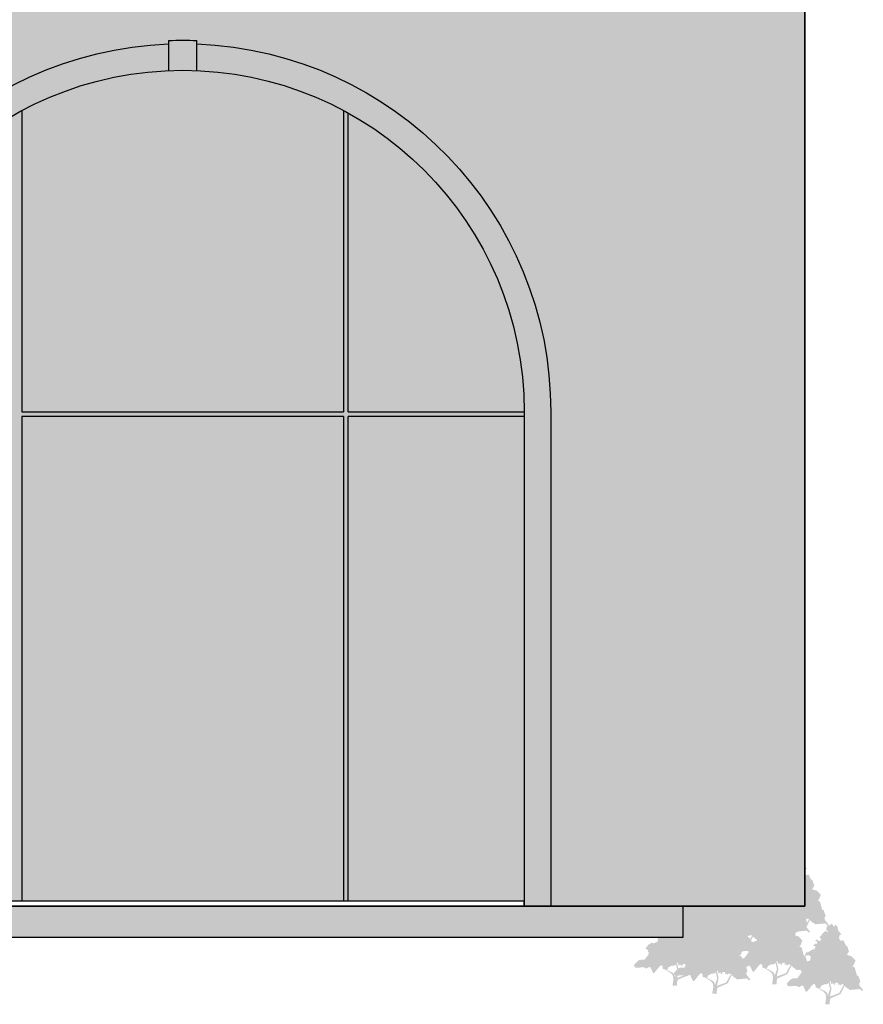
# Model space of a CAD drawing. Units: feet. Extents: x 2368 to 3224, y 836 to 1229.
# Tile 7 of 9: x 2603 to 2728, y 839 to 985. Entities that reach past the tile are written whole.
import ezdxf

# ---------------------------------------------------------------- set-up
doc = ezdxf.new("R2010")
doc.units = ezdxf.units.FT
for name, color, linetype, lineweight in [('A-ELEV', 7, 'Continuous', 25), ('A-ELEV-PATT', 8, 'Continuous', 13), ('L-PLNT', 3, 'Continuous', 13)]:
    doc.layers.add(name, color=color, linetype=linetype, lineweight=lineweight)

msp = doc.modelspace()

# ---------------------------------------------------------------- hatches: boundary and pattern name
at = {"layer": 'A-ELEV-PATT'}
h = msp.add_hatch(color=256, dxfattribs=at)
h.dxf.hatch_style = 1
h.paths.add_polyline_path([(2582.11, 1191.22), (2544.98, 1191.22), (2544.98, 1108.75), (2582.11, 1108.75)])
h.paths.add_polyline_path([(2653.72, 1191.22), (2584.6, 1191.22), (2584.6, 1108.75), (2653.72, 1108.75)])
h.paths.add_polyline_path([(2693.73, 1191.22), (2656.21, 1191.22), (2656.21, 1108.75), (2693.73, 1108.75)])
h.paths.add_polyline_path([(2653.72, 1099.51), (2584.6, 1099.51), (2584.6, 1040.78), (2653.72, 1040.78)])
h.paths.add_polyline_path([(2693.73, 1099.51), (2656.21, 1099.51), (2656.21, 1040.78), (2693.73, 1040.78)])
h.paths.add_polyline_path([(2582.11, 1099.51), (2544.98, 1099.51), (2544.98, 1040.78), (2582.11, 1040.78)])
h.paths.add_polyline_path([(2582.11, 1036.77), (2544.98, 1036.77), (2544.98, 1033.48), (2582.11, 1033.48)])
h.paths.add_polyline_path([(2582.11, 1033.11), (2544.98, 1033.11), (2544.98, 1029.83), (2582.11, 1029.83)])
h.paths.add_polyline_path([(2582.11, 1029.46), (2544.98, 1029.46), (2544.98, 1026.18), (2582.11, 1026.18)])
h.paths.add_polyline_path([(2582.11, 1025.81), (2544.98, 1025.81), (2544.98, 1022.52), (2582.11, 1022.52)])
h.paths.add_polyline_path([(2582.11, 1022.15), (2544.98, 1022.15), (2544.98, 1018.87), (2582.11, 1018.87)])
h.paths.add_polyline_path([(2582.11, 1018.5), (2544.98, 1018.5), (2544.98, 1015.21), (2582.11, 1015.21)])
h.paths.add_polyline_path([(2582.11, 1007.53), (2544.98, 1007.53), (2544.98, 1006.11), (2582.11, 1006.11)])
h.paths.add_polyline_path([(2582.11, 1011.19), (2544.98, 1011.19), (2544.98, 1007.9), (2582.11, 1007.9)])
h.paths.add_polyline_path([(2582.11, 1014.84), (2544.98, 1014.84), (2544.98, 1011.56), (2582.11, 1011.56)])
h.paths.add_polyline_path([(2619.49, 1007.53), (2584.6, 1007.53), (2584.6, 1006.11), (2619.49, 1006.11)])
h.paths.add_polyline_path([(2619.49, 1011.19), (2584.6, 1011.19), (2584.6, 1007.9), (2619.49, 1007.9)])
h.paths.add_polyline_path([(2619.49, 1014.84), (2584.6, 1014.84), (2584.6, 1011.56), (2619.49, 1011.56)])
h.paths.add_polyline_path([(2619.49, 1018.5), (2584.6, 1018.5), (2584.6, 1015.21), (2619.49, 1015.21)])
h.paths.add_polyline_path([(2619.49, 1022.15), (2584.6, 1022.15), (2584.6, 1018.87), (2619.49, 1018.87)])
h.paths.add_polyline_path([(2619.49, 1025.81), (2584.6, 1025.81), (2584.6, 1022.52), (2619.49, 1022.52)])
h.paths.add_polyline_path([(2619.49, 1029.46), (2584.6, 1029.46), (2584.6, 1026.18), (2619.49, 1026.18)])
h.paths.add_polyline_path([(2619.49, 1033.11), (2584.6, 1033.11), (2584.6, 1029.83), (2619.49, 1029.83)])
h.paths.add_polyline_path([(2619.49, 1036.77), (2584.6, 1036.77), (2584.6, 1033.48), (2619.49, 1033.48)])
h.paths.add_polyline_path([(2582.11, 1040.06), (2544.98, 1040.06), (2544.98, 1037.14), (2582.11, 1037.14)])
h.paths.add_polyline_path([(2619.49, 1040.06), (2584.6, 1040.06), (2584.6, 1037.14), (2619.49, 1037.14)])
h.paths.add_polyline_path([(2653.72, 1040.06), (2620.43, 1040.06), (2620.43, 1037.14), (2653.72, 1037.14)])
h.paths.add_polyline_path([(2653.72, 1036.77), (2620.43, 1036.77), (2620.43, 1033.48), (2653.72, 1033.48)])
h.paths.add_polyline_path([(2653.72, 1033.11), (2620.43, 1033.11), (2620.43, 1029.83), (2653.72, 1029.83)])
h.paths.add_polyline_path([(2653.72, 1029.46), (2620.43, 1029.46), (2620.43, 1026.18), (2653.72, 1026.18)])
h.paths.add_polyline_path([(2653.72, 1025.81), (2620.43, 1025.81), (2620.43, 1022.52), (2653.72, 1022.52)])
h.paths.add_polyline_path([(2653.72, 1022.15), (2620.43, 1022.15), (2620.43, 1018.87), (2653.72, 1018.87)])
h.paths.add_polyline_path([(2653.72, 1018.5), (2620.43, 1018.5), (2620.43, 1015.21), (2653.72, 1015.21)])
h.paths.add_polyline_path([(2653.72, 1011.19), (2620.43, 1011.19), (2620.43, 1007.9), (2653.72, 1007.9)])
h.paths.add_polyline_path([(2653.72, 1014.84), (2620.43, 1014.84), (2620.43, 1011.56), (2653.72, 1011.56)])
h.paths.add_polyline_path([(2653.72, 1007.53), (2620.43, 1007.53), (2620.43, 1006.11), (2653.72, 1006.11)])
h.paths.add_polyline_path([(2693.73, 1007.53), (2656.21, 1007.53), (2656.21, 1006.11), (2693.73, 1006.11)])
h.paths.add_polyline_path([(2693.73, 1011.19), (2656.21, 1011.19), (2656.21, 1007.9), (2693.73, 1007.9)])
h.paths.add_polyline_path([(2693.73, 1014.84), (2656.21, 1014.84), (2656.21, 1011.56), (2693.73, 1011.56)])
h.paths.add_polyline_path([(2693.73, 1018.5), (2656.21, 1018.5), (2656.21, 1015.21), (2693.73, 1015.21)])
h.paths.add_polyline_path([(2693.73, 1022.15), (2656.21, 1022.15), (2656.21, 1018.87), (2693.73, 1018.87)])
h.paths.add_polyline_path([(2693.73, 1025.81), (2656.21, 1025.81), (2656.21, 1022.52), (2693.73, 1022.52)])
h.paths.add_polyline_path([(2693.73, 1029.46), (2656.21, 1029.46), (2656.21, 1026.18), (2693.73, 1026.18)])
h.paths.add_polyline_path([(2693.73, 1033.11), (2656.21, 1033.11), (2656.21, 1029.83), (2693.73, 1029.83)])
h.paths.add_polyline_path([(2693.73, 1040.06), (2656.21, 1040.06), (2656.21, 1037.14), (2693.73, 1037.14)])
h.paths.add_polyline_path([(2693.73, 1036.77), (2656.21, 1036.77), (2656.21, 1033.48), (2693.73, 1033.48)])
h.paths.add_polyline_path([(2510.02, 968.65), (2451.35, 968.65), (2451.35, 916.99), (2510.02, 916.99)])
h.paths.add_polyline_path([(2510.02, 916.99), (2470.8, 916.99), (2470.8, 861.76), (2510.02, 861.76)])
h.paths.add_polyline_path([(2650.82, 971.36, 0.250141), (2603.19, 971.36), (2603.19, 926.73), (2650.82, 926.73)])
h.paths.add_polyline_path([(2651.5, 971), (2651.5, 926.73), (2677.6, 926.73, 0.272847)])
h.paths.add_polyline_path([(2677.6, 926.06), (2651.5, 926.06), (2651.5, 854.24), (2677.6, 854.24)])
h.paths.add_polyline_path([(2650.82, 926.06), (2603.19, 926.06), (2603.19, 854.24), (2650.82, 854.24)])
h.paths.add_polyline_path([(2602.51, 971, 0.272847), (2576.42, 926.73), (2602.51, 926.73)])
h.paths.add_polyline_path([(2602.51, 926.06), (2576.42, 926.06), (2576.42, 854.24), (2602.51, 854.24)])
h = msp.add_hatch(color=256, dxfattribs=at)
h.dxf.hatch_style = 1
h.paths.add_polyline_path([(2624.92, 981.22), (2624.92, 981.73, -0.018787), (2629.09, 981.73), (2629.09, 981.22, -0.403049), (2681.53, 926.73), (2681.53, 853.51), (2701.14, 853.51), (2719.16, 853.51), (2719.16, 987.86), (2694.93, 987.86), (2544.98, 987.86), (2510.02, 987.86), (2510.02, 853.51), (2520.58, 853.51), (2520.05, 853.96), (2521, 855.17), (2521.51, 855.27), (2521.73, 855.83), (2522.31, 855.46), (2523.63, 855.92), (2523.84, 857.04), (2523.12, 857.51), (2521.95, 857.23), (2522.6, 858.63), (2522.68, 858.26), (2523.55, 858.73), (2524.28, 859.19), (2524.94, 859.29), (2525.23, 860.22), (2524.5, 860.32), (2525.17, 860.97), (2525.74, 860.88), (2525.67, 861.62), (2525.16, 861.72), (2525.3, 862.09), (2525.67, 862.19), (2526.32, 861.72), (2526.98, 862.19), (2526.47, 863.03), (2526.98, 863.31), (2526.98, 863.59), (2528.51, 865.09), (2528.51, 865.74), (2528.95, 866.58), (2529.53, 866.48), (2530.04, 866.95), (2530.41, 866.77), (2530.48, 866.3), (2530.77, 866.11), (2531.28, 866.67), (2531.86, 866.03), (2532.01, 864.99), (2533.1, 863.68), (2532.52, 863.68), (2532.3, 862.65), (2532.67, 861.9), (2533.18, 861.9), (2533.61, 862), (2534.34, 860.41), (2534.71, 860.41), (2535.29, 858.63), (2534.63, 857.61), (2536.09, 857.14), (2537.26, 855.92), (2536.52, 854.02), (2536.97, 853.96), (2537.09, 853.51), (2572.48, 853.51), (2572.48, 926.73, -0.403049)])
h.paths.add_polyline_path([(2536.7, 926.19), (2536.7, 904.71), (2529.87, 904.71), (2529.87, 926.19)], flags=16)
h = msp.add_hatch(color=256, dxfattribs=at)
h.dxf.hatch_style = 1
h.paths.add_polyline_path([(2624.92, 981.22, 0.403049), (2572.48, 926.73), (2572.48, 853.51), (2576.42, 853.51), (2576.42, 926.73, -0.402184), (2624.92, 977.28)])
h.paths.add_polyline_path([(2629.09, 981.22), (2629.09, 977.28, -0.402184), (2677.6, 926.73), (2677.6, 853.51), (2681.53, 853.51), (2681.53, 926.73, 0.403049)])
h.paths.add_polyline_path([(2629.09, 981.22), (2629.09, 981.73, 0.018787), (2624.92, 981.73), (2624.92, 977.28, -0.020626), (2629.09, 977.28)])
h = msp.add_hatch(color=256, dxfattribs=at)
h.dxf.hatch_style = 1
h.paths.add_polyline_path([(2603.19, 971.36, 0.00378), (2602.51, 971), (2602.51, 926.73), (2576.42, 926.73), (2576.42, 926.06), (2602.51, 926.06), (2602.51, 854.24), (2603.19, 854.24), (2603.19, 926.06), (2650.82, 926.06), (2650.82, 854.24), (2651.5, 854.24), (2651.5, 926.06), (2677.6, 926.06), (2677.6, 926.73), (2651.5, 926.73), (2651.5, 971, 0.00378), (2650.82, 971.36), (2650.82, 926.73), (2603.19, 926.73)])
h = msp.add_hatch(color=256, dxfattribs=at)
h.dxf.hatch_style = 1
h.paths.add_polyline_path([(2701.14, 853.51), (2538.51, 853.51), (2538.51, 848.93), (2701.14, 848.93)])
at = {"layer": 'L-PLNT'}
h = msp.add_hatch(color=256, dxfattribs=at)
h.dxf.hatch_style = 1
h.paths.add_polyline_path([(2709.04, 864.51), (2707.88, 865.72), (2706.42, 866.19), (2707.07, 867.22), (2706.49, 869), (2706.13, 869), (2705.4, 870.58), (2704.96, 870.49), (2704.45, 870.49), (2704.09, 871.24), (2704.3, 872.27), (2704.89, 872.27), (2703.79, 873.58), (2703.65, 874.61), (2703.06, 875.26), (2702.55, 874.7), (2702.26, 874.88), (2702.19, 875.35), (2701.83, 875.54), (2701.31, 875.07), (2700.73, 875.16), (2700.29, 874.32), (2700.29, 873.58), (2700.88, 873.3), (2700.44, 873.01), (2700, 873.39), (2698.76, 872.17), (2698.76, 871.89), (2698.25, 871.61), (2698.4, 871.33), (2698.76, 870.77), (2698.11, 870.3), (2697.45, 870.77), (2697.09, 870.68), (2696.94, 870.3), (2697.45, 870.21), (2697.52, 869.46), (2696.95, 869.56), (2696.28, 868.9), (2697.01, 868.81), (2696.72, 867.87), (2696.07, 867.78), (2695.34, 867.31), (2694.46, 866.85), (2694.39, 867.22), (2693.73, 865.82), (2694.9, 866.1), (2695.63, 865.63), (2695.41, 864.51), (2694.1, 864.04), (2693.51, 864.42), (2693.29, 863.85), (2692.78, 863.76), (2692.35, 863.2), (2691.84, 862.55), (2692.49, 861.99), (2692.93, 862.27), (2692.44, 861.45), (2692.79, 861.49), (2692.74, 860.76), (2691.54, 859.18), (2690.09, 859.09), (2689.43, 858.71), (2688.34, 857.5), (2688.77, 856.75), (2691.47, 856.84), (2691.98, 856.47), (2693.22, 857.03), (2694.1, 855.16), (2694.46, 855.16), (2696.14, 857.22), (2696.65, 857.5), (2697.01, 857.03), (2697.01, 856.38), (2697.6, 856.19), (2698.4, 856.19), (2698.69, 856.84), (2699.64, 857.31), (2700.59, 857.41), (2701.02, 857.78), (2701.1, 857.87), (2701.31, 858.34), (2701.61, 858.15), (2701.83, 857.41), (2702.34, 857.69), (2702.48, 857.5), (2702.63, 857.03), (2703.14, 857.87), (2703.65, 857.87), (2703.87, 857.5), (2703.65, 857.12), (2704.23, 857.31), (2704.45, 857.03), (2704.96, 857.41), (2705.47, 857.22), (2706.49, 856.19), (2706.93, 856), (2707.29, 855.63), (2710.36, 855.91), (2710.94, 855.35), (2711.38, 855.54), (2710.21, 857.03), (2710.14, 857.59), (2710.5, 858.15), (2709.85, 859.93), (2709.48, 859.93), (2708.75, 862.55), (2708.02, 862.64), (2708.46, 863.01)])
h = msp.add_hatch(color=256, dxfattribs=at)
h.dxf.hatch_style = 1
h.paths.add_polyline_path([(2711.33, 856.68), (2710.76, 857.28), (2710.04, 857.51), (2710.36, 858.02), (2710.08, 858.9), (2709.9, 858.9), (2709.54, 859.68), (2709.32, 859.63), (2709.07, 859.63), (2708.89, 860), (2709, 860.51), (2709.29, 860.51), (2708.75, 861.15), (2708.67, 861.67), (2708.39, 861.98), (2708.13, 861.71), (2707.99, 861.8), (2707.96, 862.03), (2707.78, 862.12), (2707.52, 861.89), (2707.24, 861.94), (2707.02, 861.52), (2707.02, 861.15), (2707.31, 861.02), (2707.09, 860.88), (2706.88, 861.06), (2706.27, 860.46), (2706.27, 860.33), (2706.01, 860.19), (2706.09, 860.05), (2706.27, 859.77), (2705.94, 859.54), (2705.62, 859.77), (2705.44, 859.73), (2705.37, 859.54), (2705.62, 859.5), (2705.65, 859.13), (2705.37, 859.17), (2705.04, 858.85), (2705.4, 858.8), (2705.26, 858.34), (2704.94, 858.3), (2704.58, 858.07), (2704.14, 857.84), (2704.11, 858.02), (2703.79, 857.33), (2704.36, 857.47), (2704.72, 857.24), (2704.61, 856.68), (2703.97, 856.45), (2703.68, 856.64), (2703.57, 856.36), (2703.32, 856.32), (2703.1, 856.04), (2702.85, 855.72), (2703.17, 855.44), (2703.39, 855.58), (2703.15, 855.18), (2703.32, 855.2), (2703.3, 854.84), (2702.71, 854.06), (2701.99, 854.01), (2701.66, 853.83), (2701.13, 853.23), (2701.34, 852.86), (2702.67, 852.91), (2702.92, 852.72), (2703.53, 853), (2703.97, 852.08), (2704.14, 852.08), (2704.97, 853.09), (2705.22, 853.23), (2705.4, 853), (2705.4, 852.68), (2705.69, 852.58), (2706.09, 852.58), (2706.23, 852.91), (2706.7, 853.14), (2707.16, 853.18), (2707.38, 853.37), (2707.42, 853.41), (2707.52, 853.64), (2707.67, 853.55), (2707.78, 853.18), (2708.03, 853.32), (2708.1, 853.23), (2708.17, 853), (2708.42, 853.41), (2708.67, 853.41), (2708.78, 853.23), (2708.67, 853.04), (2708.96, 853.14), (2709.07, 853), (2709.32, 853.18), (2709.57, 853.09), (2710.08, 852.58), (2710.29, 852.49), (2710.47, 852.31), (2711.98, 852.45), (2712.27, 852.17), (2712.48, 852.26), (2711.91, 853), (2711.87, 853.27), (2712.05, 853.55), (2711.73, 854.43), (2711.55, 854.43), (2711.19, 855.72), (2710.83, 855.76), (2711.05, 855.95)])
h = msp.add_hatch(color=256, dxfattribs=at)
h.dxf.hatch_style = 1
h.paths.add_polyline_path([(2720.19, 856.88), (2719.61, 857.48), (2718.89, 857.71), (2719.22, 858.22), (2718.93, 859.09), (2718.75, 859.09), (2718.39, 859.88), (2718.18, 859.83), (2717.92, 859.83), (2717.74, 860.2), (2717.85, 860.71), (2718.14, 860.71), (2717.6, 861.35), (2717.53, 861.86), (2717.24, 862.18), (2716.99, 861.9), (2716.85, 862), (2716.81, 862.23), (2716.63, 862.32), (2716.38, 862.09), (2716.09, 862.13), (2715.88, 861.72), (2715.88, 861.35), (2716.16, 861.21), (2715.95, 861.07), (2715.73, 861.26), (2715.12, 860.66), (2715.12, 860.52), (2714.87, 860.38), (2714.94, 860.25), (2715.12, 859.97), (2714.8, 859.74), (2714.47, 859.97), (2714.29, 859.92), (2714.22, 859.74), (2714.47, 859.69), (2714.51, 859.32), (2714.23, 859.37), (2713.9, 859.05), (2714.26, 859), (2714.11, 858.54), (2713.79, 858.49), (2713.43, 858.26), (2713, 858.03), (2712.96, 858.22), (2712.64, 857.53), (2713.22, 857.66), (2713.57, 857.43), (2713.47, 856.88), (2712.82, 856.65), (2712.53, 856.84), (2712.42, 856.56), (2712.17, 856.51), (2711.96, 856.24), (2711.71, 855.91), (2712.03, 855.64), (2712.24, 855.78), (2712, 855.37), (2712.18, 855.4), (2712.15, 855.03), (2711.56, 854.25), (2710.84, 854.21), (2710.52, 854.02), (2709.98, 853.43), (2710.2, 853.06), (2711.53, 853.1), (2711.78, 852.92), (2712.39, 853.19), (2712.82, 852.27), (2713, 852.27), (2713.83, 853.29), (2714.08, 853.43), (2714.26, 853.19), (2714.26, 852.87), (2714.55, 852.78), (2714.94, 852.78), (2715.08, 853.1), (2715.55, 853.33), (2716.02, 853.38), (2716.23, 853.56), (2716.27, 853.61), (2716.38, 853.84), (2716.52, 853.75), (2716.63, 853.38), (2716.88, 853.52), (2716.95, 853.43), (2717.03, 853.19), (2717.28, 853.61), (2717.53, 853.61), (2717.64, 853.43), (2717.53, 853.24), (2717.82, 853.33), (2717.92, 853.19), (2718.18, 853.38), (2718.43, 853.29), (2718.93, 852.78), (2719.15, 852.69), (2719.33, 852.5), (2720.84, 852.64), (2721.12, 852.37), (2721.34, 852.46), (2720.76, 853.19), (2720.73, 853.47), (2720.91, 853.75), (2720.58, 854.62), (2720.4, 854.62), (2720.04, 855.91), (2719.69, 855.96), (2719.9, 856.14)])
h = msp.add_hatch(color=256, dxfattribs=at)
h.dxf.hatch_style = 1
h.paths.add_polyline_path([(2721.54, 855.2), (2720.97, 855.8), (2720.25, 856.03), (2720.57, 856.54), (2720.28, 857.42), (2720.1, 857.42), (2719.75, 858.2), (2719.53, 858.15), (2719.28, 858.15), (2719.1, 858.52), (2719.21, 859.03), (2719.49, 859.03), (2718.95, 859.67), (2718.88, 860.19), (2718.6, 860.5), (2718.34, 860.23), (2718.2, 860.32), (2718.16, 860.55), (2717.98, 860.64), (2717.73, 860.41), (2717.44, 860.46), (2717.23, 860.04), (2717.23, 859.67), (2717.52, 859.54), (2717.3, 859.4), (2717.09, 859.58), (2716.47, 858.98), (2716.47, 858.84), (2716.22, 858.71), (2716.29, 858.57), (2716.47, 858.29), (2716.15, 858.06), (2715.83, 858.29), (2715.65, 858.25), (2715.58, 858.06), (2715.83, 858.01), (2715.86, 857.65), (2715.58, 857.69), (2715.25, 857.37), (2715.61, 857.32), (2715.47, 856.86), (2715.14, 856.82), (2714.79, 856.59), (2714.35, 856.36), (2714.32, 856.54), (2713.99, 855.85), (2714.57, 855.99), (2714.93, 855.76), (2714.82, 855.2), (2714.17, 854.97), (2713.89, 855.16), (2713.78, 854.88), (2713.53, 854.84), (2713.31, 854.56), (2713.06, 854.24), (2713.38, 853.96), (2713.6, 854.1), (2713.35, 853.7), (2713.53, 853.72), (2713.51, 853.36), (2712.92, 852.58), (2712.2, 852.53), (2711.87, 852.35), (2711.33, 851.75), (2711.55, 851.38), (2712.88, 851.43), (2713.13, 851.24), (2713.74, 851.52), (2714.17, 850.6), (2714.35, 850.6), (2715.18, 851.61), (2715.43, 851.75), (2715.61, 851.52), (2715.61, 851.19), (2715.9, 851.1), (2716.29, 851.1), (2716.44, 851.43), (2716.91, 851.66), (2717.37, 851.7), (2717.59, 851.89), (2717.62, 851.93), (2717.73, 852.16), (2717.88, 852.07), (2717.98, 851.7), (2718.24, 851.84), (2718.31, 851.75), (2718.38, 851.52), (2718.63, 851.93), (2718.88, 851.93), (2718.99, 851.75), (2718.88, 851.56), (2719.17, 851.66), (2719.28, 851.52), (2719.53, 851.7), (2719.78, 851.61), (2720.28, 851.1), (2720.5, 851.01), (2720.68, 850.83), (2722.19, 850.96), (2722.48, 850.69), (2722.69, 850.78), (2722.12, 851.52), (2722.08, 851.79), (2722.26, 852.07), (2721.94, 852.95), (2721.76, 852.95), (2721.4, 854.24), (2721.04, 854.28), (2721.26, 854.47)])
h = msp.add_hatch(color=256, dxfattribs=at)
h.dxf.hatch_style = 1
h.paths.add_polyline_path([(2713.05, 854.43), (2712.48, 855.02), (2711.76, 855.26), (2712.08, 855.76), (2711.8, 856.64), (2711.62, 856.64), (2711.26, 857.42), (2711.04, 857.37), (2710.79, 857.37), (2710.61, 857.74), (2710.72, 858.25), (2711.01, 858.25), (2710.47, 858.9), (2710.39, 859.41), (2710.11, 859.73), (2709.86, 859.45), (2709.71, 859.54), (2709.68, 859.77), (2709.5, 859.86), (2709.24, 859.63), (2708.96, 859.68), (2708.74, 859.26), (2708.74, 858.9), (2709.03, 858.76), (2708.81, 858.62), (2708.6, 858.8), (2707.99, 858.2), (2707.99, 858.07), (2707.73, 857.93), (2707.81, 857.79), (2707.99, 857.51), (2707.66, 857.28), (2707.34, 857.51), (2707.16, 857.47), (2707.09, 857.28), (2707.34, 857.24), (2707.38, 856.87), (2707.09, 856.91), (2706.76, 856.59), (2707.12, 856.55), (2706.98, 856.08), (2706.66, 856.04), (2706.3, 855.81), (2705.87, 855.58), (2705.83, 855.76), (2705.51, 855.07), (2706.08, 855.21), (2706.44, 854.98), (2706.33, 854.43), (2705.69, 854.2), (2705.4, 854.38), (2705.29, 854.1), (2705.04, 854.06), (2704.82, 853.78), (2704.57, 853.46), (2704.9, 853.18), (2705.11, 853.32), (2704.87, 852.92), (2705.04, 852.94), (2705.02, 852.58), (2704.43, 851.8), (2703.71, 851.75), (2703.39, 851.57), (2702.85, 850.97), (2703.06, 850.6), (2704.39, 850.65), (2704.64, 850.46), (2705.25, 850.74), (2705.69, 849.82), (2705.87, 849.82), (2706.69, 850.83), (2706.94, 850.97), (2707.12, 850.74), (2707.12, 850.42), (2707.41, 850.32), (2707.81, 850.32), (2707.95, 850.65), (2708.42, 850.88), (2708.89, 850.92), (2709.1, 851.11), (2709.14, 851.15), (2709.24, 851.38), (2709.39, 851.29), (2709.5, 850.92), (2709.75, 851.06), (2709.82, 850.97), (2709.89, 850.74), (2710.14, 851.15), (2710.39, 851.15), (2710.5, 850.97), (2710.39, 850.79), (2710.68, 850.88), (2710.79, 850.74), (2711.04, 850.92), (2711.29, 850.83), (2711.8, 850.32), (2712.01, 850.23), (2712.19, 850.05), (2713.7, 850.19), (2713.99, 849.91), (2714.2, 850), (2713.63, 850.74), (2713.59, 851.02), (2713.77, 851.29), (2713.45, 852.17), (2713.27, 852.17), (2712.91, 853.46), (2712.55, 853.5), (2712.77, 853.69)])
h = msp.add_hatch(color=256, dxfattribs=at)
h.dxf.hatch_style = 1
h.paths.add_polyline_path([(2718.81, 854.13), (2718.24, 854.73), (2717.52, 854.96), (2717.84, 855.47), (2717.55, 856.34), (2717.37, 856.34), (2717.01, 857.12), (2716.8, 857.08), (2716.55, 857.08), (2716.37, 857.45), (2716.47, 857.95), (2716.76, 857.95), (2716.22, 858.6), (2716.15, 859.11), (2715.86, 859.43), (2715.61, 859.15), (2715.47, 859.24), (2715.43, 859.47), (2715.25, 859.57), (2715, 859.34), (2714.71, 859.38), (2714.5, 858.97), (2714.5, 858.6), (2714.79, 858.46), (2714.57, 858.32), (2714.35, 858.51), (2713.74, 857.91), (2713.74, 857.77), (2713.49, 857.63), (2713.56, 857.49), (2713.74, 857.22), (2713.42, 856.99), (2713.1, 857.22), (2712.92, 857.17), (2712.84, 856.99), (2713.1, 856.94), (2713.13, 856.57), (2712.85, 856.62), (2712.52, 856.29), (2712.88, 856.25), (2712.74, 855.79), (2712.41, 855.74), (2712.05, 855.51), (2711.62, 855.28), (2711.59, 855.47), (2711.26, 854.77), (2711.84, 854.91), (2712.2, 854.68), (2712.09, 854.13), (2711.44, 853.9), (2711.16, 854.08), (2711.05, 853.81), (2710.8, 853.76), (2710.58, 853.48), (2710.33, 853.16), (2710.65, 852.88), (2710.87, 853.02), (2710.62, 852.62), (2710.8, 852.64), (2710.78, 852.28), (2710.18, 851.5), (2709.47, 851.46), (2709.14, 851.27), (2708.6, 850.67), (2708.82, 850.3), (2710.15, 850.35), (2710.4, 850.17), (2711.01, 850.44), (2711.44, 849.52), (2711.62, 849.52), (2712.45, 850.53), (2712.7, 850.67), (2712.88, 850.44), (2712.88, 850.12), (2713.17, 850.03), (2713.56, 850.03), (2713.71, 850.35), (2714.17, 850.58), (2714.64, 850.63), (2714.86, 850.81), (2714.89, 850.86), (2715, 851.09), (2715.14, 851), (2715.25, 850.63), (2715.5, 850.76), (2715.58, 850.67), (2715.65, 850.44), (2715.9, 850.86), (2716.15, 850.86), (2716.26, 850.67), (2716.15, 850.49), (2716.44, 850.58), (2716.55, 850.44), (2716.8, 850.63), (2717.05, 850.53), (2717.55, 850.03), (2717.77, 849.94), (2717.95, 849.75), (2719.46, 849.89), (2719.75, 849.61), (2719.96, 849.7), (2719.39, 850.44), (2719.35, 850.72), (2719.53, 851), (2719.21, 851.87), (2719.03, 851.87), (2718.67, 853.16), (2718.31, 853.21), (2718.52, 853.39)])
h = msp.add_hatch(color=256, dxfattribs=at)
h.dxf.hatch_style = 1
h.paths.add_polyline_path([(2701.46, 853.11), (2704.52, 854.41), (2705.76, 856.93), (2705.5, 857.18), (2705.47, 857.12), (2704.09, 854.69), (2701.31, 853.67), (2701.83, 856), (2701.31, 858.15), (2701.29, 858.28), (2701.1, 857.87), (2701.02, 857.78), (2700.98, 857.74), (2701.02, 857.69), (2701.39, 855.91), (2700.73, 853.95), (2700.51, 854.69), (2699.93, 855.26), (2698.25, 856.1), (2698.11, 856.19), (2697.74, 856.19), (2699.49, 855.07), (2700.08, 854.32), (2700.22, 853.29), (2699.93, 851.33), (2701.31, 851.33), (2701.24, 851.98)])
h = msp.add_hatch(color=256, dxfattribs=at)
h.dxf.hatch_style = 1
h.paths.add_polyline_path([(2713.1, 852.75), (2712.53, 853.35), (2711.81, 853.58), (2712.13, 854.09), (2711.85, 854.96), (2711.67, 854.96), (2711.31, 855.75), (2711.09, 855.7), (2710.84, 855.7), (2710.66, 856.07), (2710.77, 856.58), (2711.06, 856.58), (2710.52, 857.22), (2710.44, 857.73), (2710.16, 858.05), (2709.91, 857.78), (2709.76, 857.87), (2709.73, 858.1), (2709.55, 858.19), (2709.29, 857.96), (2709.01, 858.01), (2708.79, 857.59), (2708.79, 857.22), (2709.08, 857.08), (2708.86, 856.95), (2708.65, 857.13), (2708.04, 856.53), (2708.04, 856.39), (2707.79, 856.25), (2707.86, 856.12), (2708.04, 855.84), (2707.71, 855.61), (2707.39, 855.84), (2707.21, 855.79), (2707.14, 855.61), (2707.39, 855.56), (2707.43, 855.19), (2707.14, 855.24), (2706.81, 854.92), (2707.17, 854.87), (2707.03, 854.41), (2706.71, 854.37), (2706.35, 854.13), (2705.92, 853.9), (2705.88, 854.09), (2705.56, 853.4), (2706.13, 853.54), (2706.49, 853.31), (2706.38, 852.75), (2705.74, 852.52), (2705.45, 852.71), (2705.34, 852.43), (2705.09, 852.38), (2704.87, 852.11), (2704.62, 851.78), (2704.95, 851.51), (2705.16, 851.65), (2704.92, 851.25), (2705.09, 851.27), (2705.07, 850.9), (2704.48, 850.13), (2703.76, 850.08), (2703.44, 849.9), (2702.9, 849.3), (2703.11, 848.93), (2704.44, 848.97), (2704.69, 848.79), (2705.3, 849.07), (2705.74, 848.14), (2705.92, 848.14), (2706.74, 849.16), (2706.99, 849.3), (2707.17, 849.07), (2707.17, 848.74), (2707.46, 848.65), (2707.86, 848.65), (2708, 848.97), (2708.47, 849.2), (2708.94, 849.25), (2709.15, 849.43), (2709.19, 849.48), (2709.29, 849.71), (2709.44, 849.62), (2709.55, 849.25), (2709.8, 849.39), (2709.87, 849.3), (2709.94, 849.07), (2710.19, 849.48), (2710.44, 849.48), (2710.55, 849.3), (2710.44, 849.11), (2710.73, 849.2), (2710.84, 849.07), (2711.09, 849.25), (2711.34, 849.16), (2711.85, 848.65), (2712.06, 848.56), (2712.24, 848.37), (2713.75, 848.51), (2714.04, 848.24), (2714.26, 848.33), (2713.68, 849.07), (2713.64, 849.34), (2713.82, 849.62), (2713.5, 850.49), (2713.32, 850.49), (2712.96, 851.78), (2712.6, 851.83), (2712.82, 852.02)])
h = msp.add_hatch(color=256, dxfattribs=at)
h.dxf.hatch_style = 1
h.paths.add_polyline_path([(2706.05, 850.61), (2705.47, 851.21), (2704.75, 851.44), (2705.08, 851.95), (2704.79, 852.82), (2704.61, 852.82), (2704.25, 853.61), (2704.03, 853.56), (2703.78, 853.56), (2703.6, 853.93), (2703.71, 854.44), (2704, 854.44), (2703.46, 855.08), (2703.39, 855.59), (2703.1, 855.91), (2702.85, 855.64), (2702.7, 855.73), (2702.67, 855.96), (2702.49, 856.05), (2702.24, 855.82), (2701.95, 855.87), (2701.73, 855.45), (2701.73, 855.08), (2702.02, 854.94), (2701.8, 854.81), (2701.59, 854.99), (2700.98, 854.39), (2700.98, 854.25), (2700.73, 854.12), (2700.8, 853.98), (2700.98, 853.7), (2700.65, 853.47), (2700.33, 853.7), (2700.15, 853.65), (2700.08, 853.47), (2700.33, 853.42), (2700.37, 853.06), (2700.09, 853.1), (2699.76, 852.78), (2700.12, 852.73), (2699.97, 852.27), (2699.65, 852.23), (2699.29, 852), (2698.86, 851.77), (2698.82, 851.95), (2698.5, 851.26), (2699.07, 851.4), (2699.43, 851.17), (2699.32, 850.61), (2698.68, 850.38), (2698.39, 850.57), (2698.28, 850.29), (2698.03, 850.24), (2697.81, 849.97), (2697.56, 849.65), (2697.89, 849.37), (2698.1, 849.51), (2697.86, 849.11), (2698.04, 849.13), (2698.01, 848.76), (2697.42, 847.99), (2696.7, 847.94), (2696.38, 847.76), (2695.84, 847.16), (2696.05, 846.79), (2697.38, 846.83), (2697.64, 846.65), (2698.25, 846.93), (2698.68, 846), (2698.86, 846), (2699.68, 847.02), (2699.94, 847.16), (2700.12, 846.93), (2700.12, 846.6), (2700.4, 846.51), (2700.8, 846.51), (2700.94, 846.83), (2701.41, 847.06), (2701.88, 847.11), (2702.09, 847.3), (2702.13, 847.34), (2702.24, 847.57), (2702.38, 847.48), (2702.49, 847.11), (2702.74, 847.25), (2702.81, 847.16), (2702.88, 846.93), (2703.13, 847.34), (2703.39, 847.34), (2703.49, 847.16), (2703.39, 846.97), (2703.67, 847.06), (2703.78, 846.93), (2704.03, 847.11), (2704.28, 847.02), (2704.79, 846.51), (2705, 846.42), (2705.18, 846.24), (2706.69, 846.37), (2706.98, 846.1), (2707.2, 846.19), (2706.62, 846.93), (2706.59, 847.2), (2706.77, 847.48), (2706.44, 848.36), (2706.26, 848.36), (2705.9, 849.65), (2705.54, 849.69), (2705.76, 849.88)])
h = msp.add_hatch(color=256, dxfattribs=at)
h.dxf.hatch_style = 1
h.paths.add_polyline_path([(2710.55, 851.18), (2709.97, 851.78), (2709.25, 852.01), (2709.58, 852.52), (2709.29, 853.39), (2709.11, 853.39), (2708.75, 854.17), (2708.53, 854.13), (2708.28, 854.13), (2708.1, 854.5), (2708.21, 855), (2708.5, 855), (2707.96, 855.65), (2707.89, 856.16), (2707.6, 856.48), (2707.35, 856.2), (2707.2, 856.29), (2707.17, 856.52), (2706.99, 856.62), (2706.74, 856.39), (2706.45, 856.43), (2706.23, 856.02), (2706.23, 855.65), (2706.52, 855.51), (2706.31, 855.37), (2706.09, 855.56), (2705.48, 854.96), (2705.48, 854.82), (2705.23, 854.68), (2705.3, 854.54), (2705.48, 854.27), (2705.16, 854.04), (2704.83, 854.27), (2704.65, 854.22), (2704.58, 854.04), (2704.83, 853.99), (2704.87, 853.62), (2704.59, 853.67), (2704.26, 853.35), (2704.62, 853.3), (2704.47, 852.84), (2704.15, 852.79), (2703.79, 852.56), (2703.36, 852.33), (2703.32, 852.52), (2703, 851.82), (2703.57, 851.96), (2703.93, 851.73), (2703.83, 851.18), (2703.18, 850.95), (2702.89, 851.13), (2702.78, 850.86), (2702.53, 850.81), (2702.32, 850.53), (2702.06, 850.21), (2702.39, 849.94), (2702.6, 850.07), (2702.36, 849.67), (2702.54, 849.69), (2702.51, 849.33), (2701.92, 848.55), (2701.2, 848.51), (2700.88, 848.32), (2700.34, 847.72), (2700.55, 847.35), (2701.88, 847.4), (2702.14, 847.22), (2702.75, 847.49), (2703.18, 846.57), (2703.36, 846.57), (2704.18, 847.59), (2704.44, 847.72), (2704.62, 847.49), (2704.62, 847.17), (2704.9, 847.08), (2705.3, 847.08), (2705.44, 847.4), (2705.91, 847.63), (2706.38, 847.68), (2706.59, 847.86), (2706.63, 847.91), (2706.74, 848.14), (2706.88, 848.05), (2706.99, 847.68), (2707.24, 847.82), (2707.31, 847.72), (2707.38, 847.49), (2707.64, 847.91), (2707.89, 847.91), (2707.99, 847.72), (2707.89, 847.54), (2708.17, 847.63), (2708.28, 847.49), (2708.53, 847.68), (2708.79, 847.59), (2709.29, 847.08), (2709.5, 846.99), (2709.68, 846.8), (2711.19, 846.94), (2711.48, 846.66), (2711.7, 846.76), (2711.12, 847.49), (2711.09, 847.77), (2711.27, 848.05), (2710.94, 848.92), (2710.76, 848.92), (2710.4, 850.21), (2710.04, 850.26), (2710.26, 850.44)])
h = msp.add_hatch(color=256, dxfattribs=at)
h.dxf.hatch_style = 1
h.paths.add_polyline_path([(2704.05, 848.23), (2703.48, 848.83), (2702.76, 849.06), (2703.08, 849.57), (2702.8, 850.44), (2702.62, 850.44), (2702.26, 851.23), (2702.04, 851.18), (2701.79, 851.18), (2701.61, 851.55), (2701.72, 852.06), (2702, 852.06), (2701.47, 852.7), (2701.39, 853.21), (2701.11, 853.53), (2700.85, 853.25), (2700.71, 853.35), (2700.67, 853.58), (2700.49, 853.67), (2700.24, 853.44), (2699.96, 853.48), (2699.74, 853.07), (2699.74, 852.7), (2700.03, 852.56), (2699.81, 852.42), (2699.6, 852.61), (2698.99, 852.01), (2698.99, 851.87), (2698.73, 851.73), (2698.81, 851.59), (2698.99, 851.32), (2698.66, 851.09), (2698.34, 851.32), (2698.16, 851.27), (2698.09, 851.09), (2698.34, 851.04), (2698.37, 850.67), (2698.09, 850.72), (2697.76, 850.4), (2698.12, 850.35), (2697.98, 849.89), (2697.66, 849.84), (2697.3, 849.61), (2696.86, 849.38), (2696.83, 849.57), (2696.5, 848.88), (2697.08, 849.01), (2697.44, 848.78), (2697.33, 848.23), (2696.68, 848), (2696.4, 848.18), (2696.29, 847.91), (2696.04, 847.86), (2695.82, 847.59), (2695.57, 847.26), (2695.89, 846.99), (2696.11, 847.12), (2695.87, 846.72), (2696.04, 846.74), (2696.02, 846.38), (2695.43, 845.6), (2694.71, 845.56), (2694.38, 845.37), (2693.84, 844.77), (2694.06, 844.41), (2695.39, 844.45), (2695.64, 844.27), (2696.25, 844.54), (2696.68, 843.62), (2696.86, 843.62), (2697.69, 844.64), (2697.94, 844.77), (2698.12, 844.54), (2698.12, 844.22), (2698.41, 844.13), (2698.81, 844.13), (2698.95, 844.45), (2699.42, 844.68), (2699.88, 844.73), (2700.1, 844.91), (2700.14, 844.96), (2700.24, 845.19), (2700.39, 845.1), (2700.49, 844.73), (2700.75, 844.87), (2700.82, 844.77), (2700.89, 844.54), (2701.14, 844.96), (2701.39, 844.96), (2701.5, 844.77), (2701.39, 844.59), (2701.68, 844.68), (2701.79, 844.54), (2702.04, 844.73), (2702.29, 844.64), (2702.8, 844.13), (2703.01, 844.04), (2703.19, 843.85), (2704.7, 843.99), (2704.99, 843.71), (2705.2, 843.81), (2704.63, 844.54), (2704.59, 844.82), (2704.77, 845.1), (2704.45, 845.97), (2704.27, 845.97), (2703.91, 847.26), (2703.55, 847.31), (2703.77, 847.49)])
h = msp.add_hatch(color=256, dxfattribs=at)
h.dxf.hatch_style = 1
h.paths.add_polyline_path([(2707.6, 851.06), (2709.11, 851.71), (2709.71, 852.95), (2709.59, 853.07), (2709.57, 853.04), (2708.89, 851.85), (2707.52, 851.34), (2707.78, 852.49), (2707.52, 853.55), (2707.51, 853.61), (2707.42, 853.41), (2707.38, 853.37), (2707.36, 853.35), (2707.38, 853.32), (2707.56, 852.45), (2707.24, 851.48), (2707.13, 851.85), (2706.84, 852.12), (2706.01, 852.54), (2705.94, 852.58), (2705.76, 852.58), (2706.63, 852.03), (2706.91, 851.66), (2706.98, 851.15), (2706.84, 850.19), (2707.52, 850.19), (2707.49, 850.51)])
h = msp.add_hatch(color=256, dxfattribs=at)
h.dxf.hatch_style = 1
h.paths.add_polyline_path([(2718.81, 848.43), (2718.24, 849.03), (2717.52, 849.26), (2717.84, 849.76), (2717.55, 850.64), (2717.37, 850.64), (2717.01, 851.42), (2716.8, 851.38), (2716.55, 851.38), (2716.37, 851.74), (2716.47, 852.25), (2716.76, 852.25), (2716.22, 852.9), (2716.15, 853.41), (2715.86, 853.73), (2715.61, 853.45), (2715.47, 853.54), (2715.43, 853.77), (2715.25, 853.86), (2715, 853.63), (2714.71, 853.68), (2714.5, 853.27), (2714.5, 852.9), (2714.79, 852.76), (2714.57, 852.62), (2714.35, 852.8), (2713.74, 852.21), (2713.74, 852.07), (2713.49, 851.93), (2713.56, 851.79), (2713.74, 851.51), (2713.42, 851.28), (2713.1, 851.51), (2712.92, 851.47), (2712.84, 851.28), (2713.1, 851.24), (2713.13, 850.87), (2712.85, 850.92), (2712.52, 850.59), (2712.88, 850.55), (2712.74, 850.09), (2712.41, 850.04), (2712.05, 849.81), (2711.62, 849.58), (2711.59, 849.76), (2711.26, 849.07), (2711.84, 849.21), (2712.2, 848.98), (2712.09, 848.43), (2711.44, 848.2), (2711.16, 848.38), (2711.05, 848.1), (2710.8, 848.06), (2710.58, 847.78), (2710.33, 847.46), (2710.65, 847.18), (2710.87, 847.32), (2710.62, 846.92), (2710.8, 846.94), (2710.78, 846.58), (2710.18, 845.8), (2709.47, 845.75), (2709.14, 845.57), (2708.6, 844.97), (2708.82, 844.6), (2710.15, 844.65), (2710.4, 844.46), (2711.01, 844.74), (2711.44, 843.82), (2711.62, 843.82), (2712.45, 844.83), (2712.7, 844.97), (2712.88, 844.74), (2712.88, 844.42), (2713.17, 844.33), (2713.56, 844.33), (2713.71, 844.65), (2714.17, 844.88), (2714.64, 844.92), (2714.86, 845.11), (2714.89, 845.16), (2715, 845.39), (2715.14, 845.29), (2715.25, 844.92), (2715.5, 845.06), (2715.58, 844.97), (2715.65, 844.74), (2715.9, 845.16), (2716.15, 845.16), (2716.26, 844.97), (2716.15, 844.79), (2716.44, 844.88), (2716.55, 844.74), (2716.8, 844.92), (2717.05, 844.83), (2717.55, 844.33), (2717.77, 844.23), (2717.95, 844.05), (2719.46, 844.19), (2719.75, 843.91), (2719.96, 844), (2719.39, 844.74), (2719.35, 845.02), (2719.53, 845.29), (2719.21, 846.17), (2719.03, 846.17), (2718.67, 847.46), (2718.31, 847.51), (2718.52, 847.69)])
h = msp.add_hatch(color=256, dxfattribs=at)
h.dxf.hatch_style = 1
h.paths.add_polyline_path([(2716.45, 851.26), (2717.96, 851.9), (2718.57, 853.14), (2718.44, 853.27), (2718.43, 853.24), (2717.74, 852.04), (2716.38, 851.54), (2716.63, 852.69), (2716.38, 853.75), (2716.36, 853.81), (2716.27, 853.61), (2716.23, 853.56), (2716.21, 853.54), (2716.23, 853.52), (2716.41, 852.64), (2716.09, 851.67), (2715.98, 852.04), (2715.7, 852.32), (2714.87, 852.73), (2714.8, 852.78), (2714.62, 852.78), (2715.48, 852.23), (2715.77, 851.86), (2715.84, 851.35), (2715.7, 850.38), (2716.38, 850.38), (2716.34, 850.71)])
h = msp.add_hatch(color=256, dxfattribs=at)
h.dxf.hatch_style = 1
h.paths.add_polyline_path([(2709.96, 847.05), (2709.38, 847.65), (2708.66, 847.88), (2708.99, 848.39), (2708.7, 849.26), (2708.52, 849.26), (2708.16, 850.05), (2707.94, 850), (2707.69, 850), (2707.51, 850.37), (2707.62, 850.88), (2707.91, 850.88), (2707.37, 851.52), (2707.3, 852.03), (2707.01, 852.35), (2706.76, 852.07), (2706.61, 852.17), (2706.58, 852.4), (2706.4, 852.49), (2706.15, 852.26), (2705.86, 852.3), (2705.64, 851.89), (2705.64, 851.52), (2705.93, 851.38), (2705.71, 851.24), (2705.5, 851.43), (2704.89, 850.83), (2704.89, 850.69), (2704.64, 850.55), (2704.71, 850.41), (2704.89, 850.14), (2704.56, 849.91), (2704.24, 850.14), (2704.06, 850.09), (2703.99, 849.91), (2704.24, 849.86), (2704.28, 849.49), (2704, 849.54), (2703.67, 849.22), (2704.03, 849.17), (2703.88, 848.71), (2703.56, 848.66), (2703.2, 848.43), (2702.77, 848.2), (2702.73, 848.39), (2702.41, 847.7), (2702.98, 847.83), (2703.34, 847.6), (2703.23, 847.05), (2702.59, 846.82), (2702.3, 847), (2702.19, 846.73), (2701.94, 846.68), (2701.73, 846.41), (2701.47, 846.08), (2701.8, 845.81), (2702.01, 845.94), (2701.77, 845.54), (2701.95, 845.56), (2701.92, 845.2), (2701.33, 844.42), (2700.61, 844.38), (2700.29, 844.19), (2699.75, 843.59), (2699.96, 843.23), (2701.29, 843.27), (2701.55, 843.09), (2702.16, 843.36), (2702.59, 842.44), (2702.77, 842.44), (2703.59, 843.46), (2703.85, 843.59), (2704.03, 843.36), (2704.03, 843.04), (2704.31, 842.95), (2704.71, 842.95), (2704.85, 843.27), (2705.32, 843.5), (2705.79, 843.55), (2706, 843.73), (2706.04, 843.78), (2706.15, 844.01), (2706.29, 843.92), (2706.4, 843.55), (2706.65, 843.69), (2706.72, 843.59), (2706.79, 843.36), (2707.04, 843.78), (2707.3, 843.78), (2707.4, 843.59), (2707.3, 843.41), (2707.58, 843.5), (2707.69, 843.36), (2707.94, 843.55), (2708.2, 843.46), (2708.7, 842.95), (2708.91, 842.86), (2709.09, 842.67), (2710.6, 842.81), (2710.89, 842.53), (2711.11, 842.63), (2710.53, 843.36), (2710.5, 843.64), (2710.68, 843.92), (2710.35, 844.79), (2710.17, 844.79), (2709.81, 846.08), (2709.45, 846.13), (2709.67, 846.31)])
h = msp.add_hatch(color=256, dxfattribs=at)
h.dxf.hatch_style = 1
h.paths.add_polyline_path([(2717.8, 849.58), (2719.31, 850.23), (2719.92, 851.47), (2719.8, 851.59), (2719.78, 851.56), (2719.1, 850.37), (2717.73, 849.86), (2717.98, 851.01), (2717.73, 852.07), (2717.72, 852.13), (2717.62, 851.93), (2717.59, 851.89), (2717.57, 851.87), (2717.59, 851.84), (2717.77, 850.96), (2717.44, 850), (2717.34, 850.37), (2717.05, 850.64), (2716.22, 851.06), (2716.15, 851.1), (2715.97, 851.1), (2716.83, 850.55), (2717.12, 850.18), (2717.19, 849.67), (2717.05, 848.71), (2717.73, 848.71), (2717.7, 849.03)])
h = msp.add_hatch(color=256, dxfattribs=at)
h.dxf.hatch_style = 1
h.paths.add_polyline_path([(2709.32, 848.8), (2710.83, 849.45), (2711.43, 850.69), (2711.31, 850.81), (2711.29, 850.79), (2710.61, 849.59), (2709.24, 849.08), (2709.5, 850.23), (2709.24, 851.29), (2709.23, 851.35), (2709.14, 851.15), (2709.1, 851.11), (2709.08, 851.09), (2709.1, 851.06), (2709.28, 850.19), (2708.96, 849.22), (2708.85, 849.59), (2708.56, 849.86), (2707.73, 850.28), (2707.66, 850.32), (2707.48, 850.32), (2708.35, 849.77), (2708.63, 849.4), (2708.71, 848.9), (2708.56, 847.93), (2709.24, 847.93), (2709.21, 848.25)])
h = msp.add_hatch(color=256, dxfattribs=at)
h.dxf.hatch_style = 1
h.paths.add_polyline_path([(2715.07, 848.51), (2716.58, 849.15), (2717.19, 850.39), (2717.07, 850.52), (2717.05, 850.49), (2716.37, 849.29), (2715, 848.78), (2715.25, 849.94), (2715, 851), (2714.99, 851.06), (2714.89, 850.86), (2714.86, 850.81), (2714.83, 850.79), (2714.86, 850.76), (2715.04, 849.89), (2714.71, 848.92), (2714.61, 849.29), (2714.32, 849.57), (2713.49, 849.98), (2713.42, 850.03), (2713.24, 850.03), (2714.1, 849.47), (2714.39, 849.11), (2714.46, 848.6), (2714.32, 847.63), (2715, 847.63), (2714.97, 847.95)])
h = msp.add_hatch(color=256, dxfattribs=at)
h.dxf.hatch_style = 1
h.paths.add_polyline_path([(2726.68, 845.48), (2726.11, 846.08), (2725.39, 846.31), (2725.71, 846.81), (2725.42, 847.69), (2725.24, 847.69), (2724.88, 848.47), (2724.67, 848.43), (2724.42, 848.43), (2724.24, 848.8), (2724.35, 849.3), (2724.63, 849.3), (2724.09, 849.95), (2724.02, 850.46), (2723.73, 850.78), (2723.48, 850.5), (2723.34, 850.59), (2723.3, 850.82), (2723.12, 850.92), (2722.87, 850.68), (2722.58, 850.73), (2722.37, 850.32), (2722.37, 849.95), (2722.66, 849.81), (2722.44, 849.67), (2722.23, 849.86), (2721.61, 849.26), (2721.61, 849.12), (2721.36, 848.98), (2721.43, 848.84), (2721.61, 848.57), (2721.29, 848.33), (2720.97, 848.57), (2720.79, 848.52), (2720.72, 848.33), (2720.97, 848.29), (2721, 847.92), (2720.72, 847.97), (2720.39, 847.64), (2720.75, 847.6), (2720.61, 847.14), (2720.28, 847.09), (2719.92, 846.86), (2719.49, 846.63), (2719.46, 846.81), (2719.13, 846.12), (2719.71, 846.26), (2720.07, 846.03), (2719.96, 845.48), (2719.31, 845.25), (2719.03, 845.43), (2718.92, 845.16), (2718.67, 845.11), (2718.45, 844.83), (2718.2, 844.51), (2718.52, 844.23), (2718.74, 844.37), (2718.49, 843.97), (2718.67, 843.99), (2718.65, 843.63), (2718.06, 842.85), (2717.34, 842.8), (2717.01, 842.62), (2716.47, 842.02), (2716.69, 841.65), (2718.02, 841.7), (2718.27, 841.51), (2718.88, 841.79), (2719.31, 840.87), (2719.49, 840.87), (2720.32, 841.88), (2720.57, 842.02), (2720.75, 841.79), (2720.75, 841.47), (2721.04, 841.38), (2721.43, 841.38), (2721.58, 841.7), (2722.05, 841.93), (2722.51, 841.98), (2722.73, 842.16), (2722.76, 842.21), (2722.87, 842.44), (2723.02, 842.34), (2723.12, 841.98), (2723.38, 842.11), (2723.45, 842.02), (2723.52, 841.79), (2723.77, 842.21), (2724.02, 842.21), (2724.13, 842.02), (2724.02, 841.84), (2724.31, 841.93), (2724.42, 841.79), (2724.67, 841.98), (2724.92, 841.88), (2725.42, 841.38), (2725.64, 841.28), (2725.82, 841.1), (2727.33, 841.24), (2727.62, 840.96), (2727.83, 841.05), (2727.26, 841.79), (2727.22, 842.07), (2727.4, 842.34), (2727.08, 843.22), (2726.9, 843.22), (2726.54, 844.51), (2726.18, 844.56), (2726.39, 844.74)])
h = msp.add_hatch(color=256, dxfattribs=at)
h.dxf.hatch_style = 1
h.paths.add_polyline_path([(2709.37, 847.13), (2710.88, 847.78), (2711.49, 849.02), (2711.36, 849.14), (2711.34, 849.11), (2710.66, 847.91), (2709.29, 847.41), (2709.55, 848.56), (2709.29, 849.62), (2709.28, 849.68), (2709.19, 849.48), (2709.15, 849.43), (2709.13, 849.42), (2709.15, 849.39), (2709.33, 848.51), (2709.01, 847.55), (2708.9, 847.91), (2708.61, 848.19), (2707.79, 848.61), (2707.71, 848.65), (2707.53, 848.65), (2708.4, 848.1), (2708.68, 847.73), (2708.76, 847.22), (2708.61, 846.25), (2709.29, 846.25), (2709.26, 846.58)])
h = msp.add_hatch(color=256, dxfattribs=at)
h.dxf.hatch_style = 1
h.paths.add_polyline_path([(2702.31, 844.99), (2703.82, 845.64), (2704.43, 846.88), (2704.3, 847), (2704.28, 846.97), (2703.6, 845.77), (2702.24, 845.27), (2702.49, 846.42), (2702.24, 847.48), (2702.22, 847.54), (2702.13, 847.34), (2702.09, 847.3), (2702.07, 847.28), (2702.09, 847.25), (2702.27, 846.37), (2701.95, 845.41), (2701.84, 845.77), (2701.55, 846.05), (2700.73, 846.47), (2700.66, 846.51), (2700.47, 846.51), (2701.34, 845.96), (2701.62, 845.59), (2701.7, 845.08), (2701.55, 844.12), (2702.24, 844.12), (2702.2, 844.44)])
h = msp.add_hatch(color=256, dxfattribs=at)
h.dxf.hatch_style = 1
h.paths.add_polyline_path([(2706.81, 845.56), (2708.32, 846.2), (2708.93, 847.44), (2708.8, 847.57), (2708.79, 847.54), (2708.1, 846.34), (2706.74, 845.83), (2706.99, 846.99), (2706.74, 848.05), (2706.72, 848.11), (2706.63, 847.91), (2706.59, 847.86), (2706.57, 847.84), (2706.59, 847.82), (2706.77, 846.94), (2706.45, 845.97), (2706.34, 846.34), (2706.05, 846.62), (2705.23, 847.03), (2705.16, 847.08), (2704.98, 847.08), (2705.84, 846.53), (2706.13, 846.16), (2706.2, 845.65), (2706.05, 844.68), (2706.74, 844.68), (2706.7, 845)])
h = msp.add_hatch(color=256, dxfattribs=at)
h.dxf.hatch_style = 1
h.paths.add_polyline_path([(2700.32, 842.61), (2701.82, 843.25), (2702.43, 844.49), (2702.31, 844.62), (2702.29, 844.59), (2701.61, 843.39), (2700.24, 842.88), (2700.49, 844.04), (2700.24, 845.1), (2700.23, 845.16), (2700.14, 844.96), (2700.1, 844.91), (2700.08, 844.89), (2700.1, 844.87), (2700.28, 843.99), (2699.96, 843.02), (2699.85, 843.39), (2699.56, 843.67), (2698.73, 844.08), (2698.66, 844.13), (2698.48, 844.13), (2699.34, 843.58), (2699.63, 843.21), (2699.7, 842.7), (2699.56, 841.73), (2700.24, 841.73), (2700.21, 842.06)])
h = msp.add_hatch(color=256, dxfattribs=at)
h.dxf.hatch_style = 1
h.paths.add_polyline_path([(2715.07, 842.8), (2716.58, 843.45), (2717.19, 844.69), (2717.07, 844.82), (2717.05, 844.79), (2716.37, 843.59), (2715, 843.08), (2715.25, 844.23), (2715, 845.29), (2714.99, 845.35), (2714.89, 845.16), (2714.86, 845.11), (2714.83, 845.09), (2714.86, 845.06), (2715.04, 844.19), (2714.71, 843.22), (2714.61, 843.59), (2714.32, 843.86), (2713.49, 844.28), (2713.42, 844.33), (2713.24, 844.33), (2714.1, 843.77), (2714.39, 843.4), (2714.46, 842.9), (2714.32, 841.93), (2715, 841.93), (2714.97, 842.25)])
h = msp.add_hatch(color=256, dxfattribs=at)
h.dxf.hatch_style = 1
h.paths.add_polyline_path([(2706.22, 841.43), (2707.73, 842.07), (2708.34, 843.31), (2708.21, 843.44), (2708.2, 843.41), (2707.51, 842.21), (2706.15, 841.71), (2706.4, 842.86), (2706.15, 843.92), (2706.13, 843.98), (2706.04, 843.78), (2706, 843.73), (2705.98, 843.71), (2706, 843.69), (2706.18, 842.81), (2705.86, 841.84), (2705.75, 842.21), (2705.46, 842.49), (2704.64, 842.9), (2704.57, 842.95), (2704.39, 842.95), (2705.25, 842.4), (2705.54, 842.03), (2705.61, 841.52), (2705.46, 840.55), (2706.15, 840.55), (2706.11, 840.88)])
h = msp.add_hatch(color=256, dxfattribs=at)
h.dxf.hatch_style = 1
h.paths.add_polyline_path([(2722.94, 839.86), (2724.45, 840.5), (2725.06, 841.74), (2724.94, 841.87), (2724.92, 841.84), (2724.24, 840.64), (2722.87, 840.13), (2723.12, 841.28), (2722.87, 842.34), (2722.86, 842.41), (2722.76, 842.21), (2722.73, 842.16), (2722.71, 842.14), (2722.73, 842.11), (2722.91, 841.24), (2722.58, 840.27), (2722.48, 840.64), (2722.19, 840.92), (2721.36, 841.33), (2721.29, 841.38), (2721.11, 841.38), (2721.97, 840.82), (2722.26, 840.45), (2722.33, 839.95), (2722.19, 838.98), (2722.87, 838.98), (2722.84, 839.3)])

# ---------------------------------------------------------------- linework, layer by layer
at = {"layer": 'A-ELEV'}
for p, q in [((2719.16, 853.51), (2719.16, 1229.35)), ((2719.16, 853.51), (2719.16, 1229.35)), ((2537.09, 853.51), (2719.16, 853.51)), ((2537.09, 853.51), (2719.16, 853.51))]:
    msp.add_line(p, q, dxfattribs=at)
for points in [[(2521.04, 853.51), (2510.02, 853.51), (2510.02, 987.86), (2719.16, 987.86), (2719.16, 853.51), (2537.09, 853.51)], [(2521.04, 853.51), (2510.02, 853.51), (2510.02, 987.86), (2719.16, 987.86), (2719.16, 853.51), (2537.09, 853.51)], [(2624.92, 981.73), (2624.92, 977.28)], [(2624.92, 981.73), (2624.92, 977.28)], [(2629.09, 977.28), (2629.09, 981.73)], [(2629.09, 977.28), (2629.09, 981.73)], [(2603.19, 971.36), (2603.19, 926.73)], [(2603.19, 971.36), (2603.19, 926.73)], [(2650.82, 971.36), (2650.82, 926.73)], [(2650.82, 971.36), (2650.82, 926.73)], [(2651.5, 926.73), (2651.5, 971)], [(2651.5, 926.73), (2651.5, 971)], [(2603.19, 926.73), (2650.82, 926.73)], [(2603.19, 926.73), (2650.82, 926.73)], [(2603.19, 926.06), (2603.19, 854.24)], [(2650.82, 926.06), (2603.19, 926.06)], [(2650.82, 926.06), (2603.19, 926.06)], [(2603.19, 926.06), (2603.19, 854.24)], [(2650.82, 926.06), (2650.82, 854.24)], [(2650.82, 926.06), (2650.82, 854.24)], [(2651.5, 926.73), (2677.6, 926.73), (2677.6, 926.06), (2651.5, 926.06)], [(2651.5, 926.73), (2677.6, 926.73), (2677.6, 926.06), (2651.5, 926.06)], [(2651.5, 854.24), (2651.5, 926.06)], [(2651.5, 854.24), (2651.5, 926.06)]]:
    msp.add_lwpolyline(points, dxfattribs=at)
for points in [[(2624.92, 981.73, -0.018787), (2629.09, 981.73)], [(2624.92, 981.73, -0.018787), (2629.09, 981.73)], [(2572.48, 853.51), (2572.48, 926.73, -0.403049), (2624.92, 981.22, -0.403049)], [(2572.48, 853.51), (2572.48, 926.73, -0.403049), (2624.92, 981.22, -0.403049)], [(2629.09, 981.22, -0.403049), (2681.53, 926.73), (2681.53, 853.51)], [(2629.09, 981.22, -0.403049), (2681.53, 926.73), (2681.53, 853.51)], [(2576.42, 853.51), (2576.42, 926.73, -1), (2677.6, 926.73), (2677.6, 853.51)], [(2576.42, 853.51), (2576.42, 926.73, -1), (2677.6, 926.73), (2677.6, 853.51)]]:
    msp.add_lwpolyline(points, format="xyb", dxfattribs=at)
for points in [[(2701.14, 853.51), (2538.51, 853.51), (2538.51, 848.93), (2701.14, 848.93)], [(2701.14, 853.51), (2538.51, 853.51), (2538.51, 848.93), (2701.14, 848.93)], [(2576.42, 853.51), (2677.6, 853.51), (2677.6, 854.24), (2576.42, 854.24)], [(2576.42, 853.51), (2677.6, 853.51), (2677.6, 854.24), (2576.42, 854.24)]]:
    msp.add_lwpolyline(points, close=True, dxfattribs=at)

doc.saveas('drawing.dxf')
